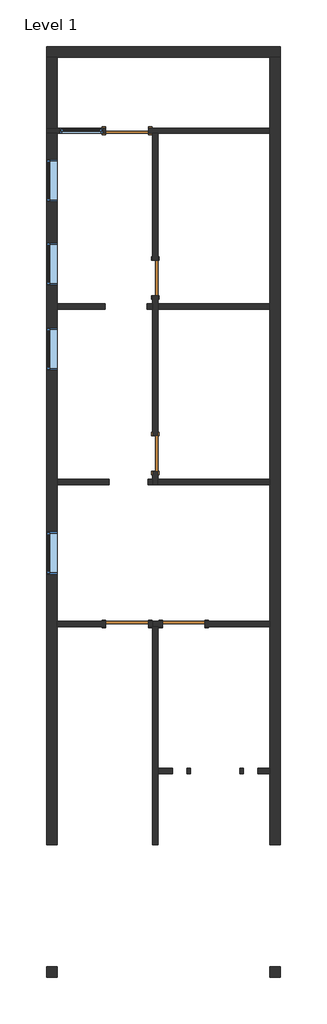
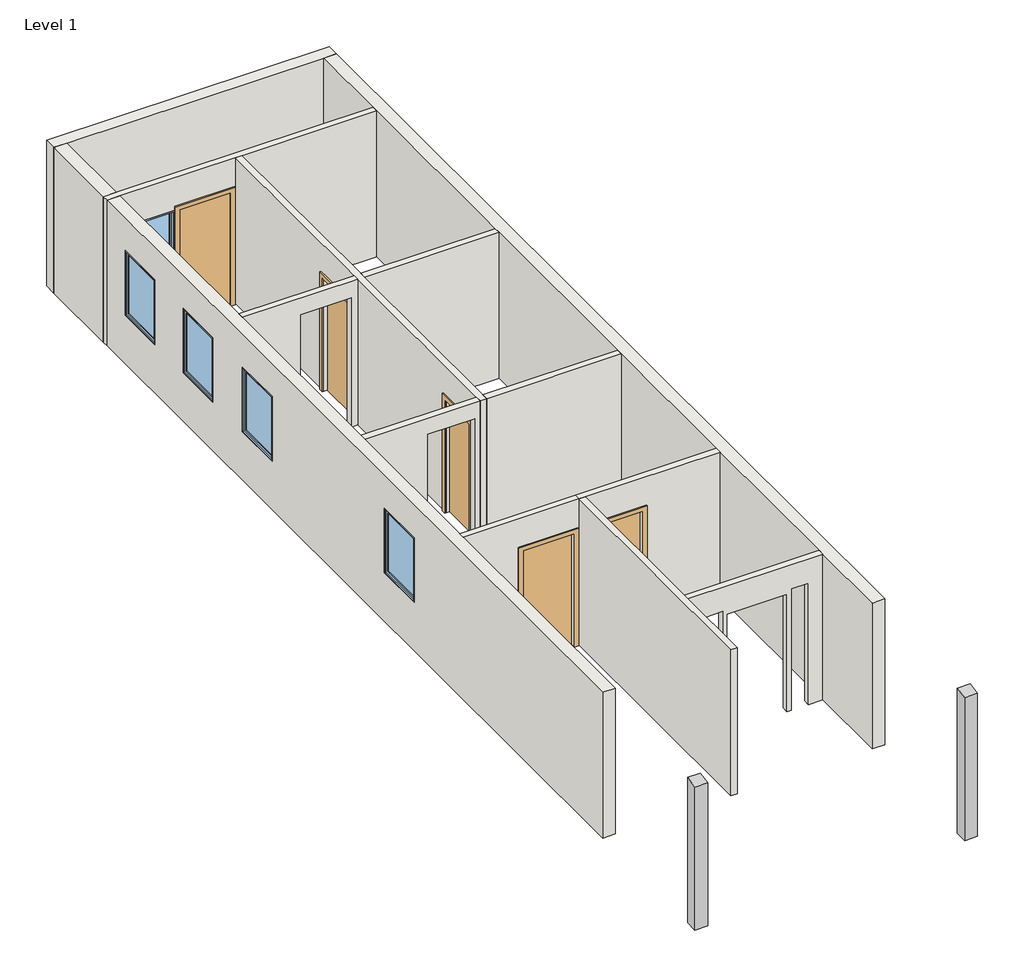
# One storey, incomplete: 14 walls, 5 doors, 5 windows, 2 columns.
"""IFC4 building model written with IfcOpenShell, lengths in millimetres."""

from ifc_helpers import new_model, si_unit, point, frame, frame_2d, origin, origin_with_axes, place, context, project, spatial, polyline, circle_curve, trimmed, segment, composite_curve, outline, extrude, faceted_brep, transform, mapped, element, save
from components import door_214872d5, door_305aa2a5, window_c1f32544, window_41a96561

model = new_model("IFC4")

# Units and contexts
model_context = context("Model", 3, world=origin())
ifc_project = project(units=[si_unit("LENGTHUNIT", "METRE", prefix="MILLI")], contexts=[model_context])

# Site, building, storey
site = spatial("IfcSite", under=ifc_project)
building = spatial("IfcBuilding", under=site)
storey = spatial("IfcBuildingStorey", under=building, Name="Level 1", Elevation=0.0)

# Columns
placement = place(None, origin())
element("IfcColumn", 1, ObjectType="Rectangular Column : 9\"X9\"", at=placement, inside=storey, context=model_context, shape_type="SweptSolid", body=[
    extrude(outline(composite_curve([segment(polyline([(-16023.0597562, 0.0), (-16251.6597562, 0.0), (-16251.6597562, 2691.3651661)]), True, "CONTINUOUS"), segment(trimmed(circle_curve(frame_2d((-13694.3342361, -9875.5261928)), 12824.4560213), [point((-16251.6597562, 2691.3651661))], [point((-16023.0597562, 2735.7271031))], False, "CARTESIAN"), True, "CONTINUOUS"), segment(polyline([(-16023.0597562, 2735.7271031), (-16023.0597562, 0.0)]), True, "CONTINUOUS")], self_intersect=False)), frame((-5651.4766939, 0.0, 0.0), z_axis=(1.0, 0.0, 0.0), x_axis=(0.0, 1.0, 0.0)), (0.0, 0.0, 1.0), 228.6),
])
element("IfcColumn", 2, ObjectType="Rectangular Column : 9\"X9\"", at=placement, inside=storey, context=model_context, shape_type="SweptSolid", body=[
    extrude(outline(composite_curve([segment(polyline([(-16023.0597562, 0.0), (-16251.6597562, 0.0), (-16251.6597562, 2691.3651661)]), True, "CONTINUOUS"), segment(trimmed(circle_curve(frame_2d((-13694.3342361, -9875.5261928)), 12824.4560213), [point((-16251.6597562, 2691.3651661))], [point((-16023.0597562, 2735.7271031))], False, "CARTESIAN"), True, "CONTINUOUS"), segment(polyline([(-16023.0597562, 2735.7271031), (-16023.0597562, 0.0)]), True, "CONTINUOUS")], self_intersect=False)), frame((-850.8766939, 0.0, 0.0), z_axis=(1.0, 0.0, 0.0), x_axis=(0.0, 1.0, 0.0)), (0.0, 0.0, 1.0), 228.6),
])

# Doors
door_shape = door_214872d5(model_context)
element("IfcDoor", 3, ObjectType="Single-Flush : 30\" x 84\"", at=placement, inside=storey, context=model_context, shape_type="MappedRepresentation", body=[
    mapped(door_shape, transform((-3308.3266939, -4999.4597562, 0.0), x_axis=(0.0, -1.0, 0.0), y_axis=(1.0, 0.0, 0.0), z_axis=(0.0, 0.0, 1.0))),
])
element("IfcDoor", 4, ObjectType="Single-Flush : 30\" x 84\"", at=placement, inside=storey, context=model_context, shape_type="MappedRepresentation", body=[
    mapped(door_shape, transform((-3308.3266939, -1227.5597562, 0.0), x_axis=(0.0, -1.0, 0.0), y_axis=(1.0, 0.0, 0.0), z_axis=(0.0, 0.0, 1.0))),
])
door_2_shape = door_305aa2a5(model_context)
element("IfcDoor", 5, ObjectType="Single-Flush : 36\" x 84\"", at=placement, inside=storey, context=model_context, shape_type="MappedRepresentation", body=[
    mapped(door_2_shape, transform((-3917.9266939, -8657.0597562, 0.0), x_axis=(-1.0, 0.0, 0.0), y_axis=(0.0, -1.0, 0.0), z_axis=(0.0, 0.0, 1.0))),
])
element("IfcDoor", 6, ObjectType="Single-Flush : 36\" x 84\"", at=placement, inside=storey, context=model_context, shape_type="MappedRepresentation", body=[
    mapped(door_2_shape, transform((-2698.7266939, -8657.0597562, 0.0), x_axis=(-1.0, 0.0, 0.0), y_axis=(0.0, -1.0, 0.0), z_axis=(0.0, 0.0, 1.0))),
])
element("IfcDoor", 7, ObjectType="Single-Flush : 36\" x 84\"", at=placement, inside=storey, context=model_context, shape_type="MappedRepresentation", body=[
    mapped(door_2_shape, transform((-3917.9266939, 1934.7402438, 0.0), x_axis=(1.0, 0.0, 0.0), y_axis=(0.0, 1.0, 0.0), z_axis=(0.0, 0.0, 1.0))),
])

# Walls
element("IfcWall", 8, ObjectType="wall 4.5\"", at=placement, inside=storey, context=model_context, shape_type="Brep", body=[
    faceted_brep([(-850.8766939, 1991.8902438, 0.0), (-3460.7266939, 1991.8902438, 0.0), (-3460.7266939, 1991.8902438, 2133.6), (-4375.1266939, 1991.8902438, 2133.6), (-4375.1266939, 1991.8902438, 0.0), (-5422.8766939, 1991.8902438, 0.0), (-5651.4766939, 1991.8902438, 0.0), (-5651.4766939, 1991.8902438, 2743.2), (-5422.8766939, 1991.8902438, 2743.2), (-850.8766939, 1991.8902438, 2743.2), (-4444.9766939, 1991.8902438, 2133.6), (-5359.3766939, 1991.8902438, 2133.6), (-5359.3766939, 1991.8902438, 914.4), (-4444.9766939, 1991.8902438, 914.4), (-3460.7266939, 1877.5902438, 2133.6), (-3460.7266939, 1877.5902438, 0.0), (-3365.4766939, 1877.5902438, 0.0), (-3251.1766939, 1877.5902438, 0.0), (-850.8766939, 1877.5902438, 0.0), (-850.8766939, 1877.5902438, 2743.2), (-3251.1766939, 1877.5902438, 2743.2), (-3365.4766939, 1877.5902438, 2743.2), (-5422.8766939, 1877.5902438, 2743.2), (-5651.4766939, 1877.5902438, 2743.2), (-5651.4766939, 1877.5902438, 0.0), (-5422.8766939, 1877.5902438, 0.0), (-4375.1266939, 1877.5902438, 0.0), (-4375.1266939, 1877.5902438, 2133.6), (-4444.9766939, 1877.5902438, 2133.6), (-4444.9766939, 1877.5902438, 914.4), (-5359.3766939, 1877.5902438, 914.4), (-5359.3766939, 1877.5902438, 2133.6)], [[[0, 1, 2, 3, 4, 5, 6, 7, 8, 9], [10, 11, 12, 13]], [[14, 15, 16, 17, 18, 19, 20, 21, 22, 23, 24, 25, 26, 27], [28, 29, 30, 31]], [[26, 25, 24, 6, 5, 4]], [[18, 17, 16, 15, 1, 0]], [[0, 9, 19, 18]], [[7, 6, 24, 23]], [[2, 1, 15, 14]], [[3, 2, 14, 27]], [[4, 3, 27, 26]], [[29, 28, 10, 13]], [[30, 29, 13, 12]], [[31, 30, 12, 11]], [[28, 31, 11, 10]], [[9, 8, 7, 23, 22, 21, 20, 19]]]),
])
element("IfcWall", 9, ObjectType="wall 4.5\"", at=placement, inside=storey, context=model_context, shape_type="Brep", body=[
    faceted_brep([(-3365.4766939, -1608.5597562, 2133.6), (-3365.4766939, -1608.5597562, 0.0), (-3365.4766939, -1780.0097562, 0.0), (-3365.4766939, -1894.3097562, 0.0), (-3365.4766939, -4618.4597562, 0.0), (-3365.4766939, -4618.4597562, 2133.6), (-3365.4766939, -5380.4597562, 2133.6), (-3365.4766939, -5380.4597562, 0.0), (-3365.4766939, -5551.9097562, 0.0), (-3365.4766939, -5666.2097562, 0.0), (-3365.4766939, -5666.2097562, 2743.2), (-3365.4766939, -5551.9097562, 2743.2), (-3365.4766939, -1894.3097562, 2743.2), (-3365.4766939, -1780.0097562, 2743.2), (-3365.4766939, 1877.5902438, 2743.2), (-3365.4766939, 1877.5902438, 0.0), (-3365.4766939, -846.5597562, 0.0), (-3365.4766939, -846.5597562, 2133.6), (-3251.1766939, -4618.4597562, 0.0), (-3251.1766939, -1894.3097562, 0.0), (-3251.1766939, -1780.0097562, 0.0), (-3251.1766939, -1608.5597562, 0.0), (-3251.1766939, -1608.5597562, 2133.6), (-3251.1766939, -846.5597562, 2133.6), (-3251.1766939, -846.5597562, 0.0), (-3251.1766939, 1877.5902438, 0.0), (-3251.1766939, 1877.5902438, 2743.2), (-3251.1766939, -1780.0097562, 2743.2), (-3251.1766939, -1894.3097562, 2743.2), (-3251.1766939, -5551.9097562, 2743.2), (-3251.1766939, -5666.2097562, 2743.2), (-3251.1766939, -5666.2097562, 0.0), (-3251.1766939, -5551.9097562, 0.0), (-3251.1766939, -5380.4597562, 0.0), (-3251.1766939, -5380.4597562, 2133.6), (-3251.1766939, -4618.4597562, 2133.6)], [[[0, 1, 2, 3, 4, 5, 6, 7, 8, 9, 10, 11, 12, 13, 14, 15, 16, 17]], [[18, 19, 20, 21, 22, 23, 24, 25, 26, 27, 28, 29, 30, 31, 32, 33, 34, 35]], [[9, 8, 7, 33, 32, 31]], [[16, 15, 25, 24]], [[4, 3, 2, 1, 21, 20, 19, 18]], [[15, 14, 26, 25]], [[10, 9, 31, 30]], [[34, 33, 7, 6]], [[35, 34, 6, 5]], [[18, 35, 5, 4]], [[22, 21, 1, 0]], [[23, 22, 0, 17]], [[24, 23, 17, 16]], [[14, 13, 12, 11, 10, 30, 29, 28, 27, 26]]]),
])
element("IfcWall", 10, ObjectType="wall 4.5\"", at=placement, inside=storey, context=model_context, shape_type="SweptSolid", body=[
    extrude(outline(polyline([(-850.8766939, -1894.3097562), (-3251.1766939, -1894.3097562), (-3251.1766939, -1780.0097562), (-850.8766939, -1780.0097562), (-850.8766939, -1894.3097562)])), origin_with_axes(), (0.0, 0.0, 1.0), 2743.2),
])
element("IfcWall", 11, ObjectType="wall 4.5\"", at=placement, inside=storey, context=model_context, shape_type="SweptSolid", body=[
    extrude(outline(polyline([(-850.8766939, -5666.2097562), (-3251.1766939, -5666.2097562), (-3251.1766939, -5551.9097562), (-850.8766939, -5551.9097562), (-850.8766939, -5666.2097562)])), origin_with_axes(), (0.0, 0.0, 1.0), 2743.2),
])
element("IfcWall", 12, ObjectType="wall 4.5\"", at=placement, inside=storey, context=model_context, shape_type="Brep", body=[
    faceted_brep([(-3365.4766939, -8714.2097562, 0.0), (-3251.1766939, -8714.2097562, 0.0), (-3155.9266939, -8714.2097562, 0.0), (-3155.9266939, -8714.2097562, 2133.6), (-2241.5266939, -8714.2097562, 2133.6), (-2241.5266939, -8714.2097562, 0.0), (-850.8766939, -8714.2097562, 0.0), (-850.8766939, -8714.2097562, 2743.2), (-3251.1766939, -8714.2097562, 2743.2), (-3365.4766939, -8714.2097562, 2743.2), (-3155.9266939, -8599.9097562, 2133.6), (-3155.9266939, -8599.9097562, 0.0), (-3365.4766939, -8599.9097562, 0.0), (-3365.4766939, -8599.9097562, 2743.2), (-850.8766939, -8599.9097562, 2743.2), (-850.8766939, -8599.9097562, 0.0), (-2241.5266939, -8599.9097562, 0.0), (-2241.5266939, -8599.9097562, 2133.6)], [[[0, 1, 2, 3, 4, 5, 6, 7, 8, 9]], [[10, 11, 12, 13, 14, 15, 16, 17]], [[16, 15, 6, 5]], [[12, 11, 2, 1, 0]], [[7, 6, 15, 14]], [[3, 2, 11, 10]], [[4, 3, 10, 17]], [[5, 4, 17, 16]], [[0, 9, 13, 12]], [[9, 8, 7, 14, 13]]]),
])
element("IfcWall", 13, ObjectType="wall 4.5\"", at=placement, inside=storey, context=model_context, shape_type="SweptSolid", body=[
    extrude(outline(polyline([(0.0, -1489.0516939), (0.0, -1412.8516939), (2286.0, -1412.8516939), (2286.0, -1108.0516939), (0.0, -1108.0516939), (0.0, -850.8766939), (2743.2, -850.8766939), (2743.2, -3251.1766939), (0.0, -3251.1766939), (0.0, -2936.8516939), (2286.0, -2936.8516939), (2286.0, -2632.0516939), (0.0, -2632.0516939), (0.0, -2555.8516939), (2209.8, -2555.8516939), (2209.8, -1489.0516939), (0.0, -1489.0516939)])), frame((0.0, -11876.5097562, 0.0), z_axis=(0.0, 1.0, 0.0), x_axis=(0.0, 0.0, 1.0)), (0.0, 0.0, 1.0), 114.3),
])
element("IfcWall", 14, ObjectType="wall 4.5\"", at=placement, inside=storey, context=model_context, shape_type="SweptSolid", body=[
    extrude(outline(polyline([(2743.2, -5422.8766939), (0.0, -5422.8766939), (0.0, -4391.959165), (2438.4, -4391.959165), (2438.4, -3483.8028016), (0.0, -3483.8028016), (0.0, -3365.4766939), (2743.2, -3365.4766939), (2743.2, -5422.8766939)])), frame((0.0, -1894.3097562, 0.0), z_axis=(0.0, 1.0, 0.0), x_axis=(0.0, 0.0, 1.0)), (0.0, 0.0, 1.0), 114.3),
])
element("IfcWall", 15, ObjectType="wall 4.5\"", at=placement, inside=storey, context=model_context, shape_type="SweptSolid", body=[
    extrude(outline(polyline([(2743.2, -5422.8766939), (0.0, -5422.8766939), (0.0, -4303.9674393), (2438.4, -4303.9674393), (2438.4, -3463.2909707), (0.0, -3463.2909707), (0.0, -3365.4766939), (2743.2, -3365.4766939), (2743.2, -5422.8766939)])), frame((0.0, -5666.2097562, 0.0), z_axis=(0.0, 1.0, 0.0), x_axis=(0.0, 0.0, 1.0)), (0.0, 0.0, 1.0), 114.3),
])
element("IfcWall", 16, ObjectType="wall 4.5\"", at=placement, inside=storey, context=model_context, shape_type="SweptSolid", body=[
    extrude(outline(polyline([(0.0, -5422.8766939), (0.0, -4375.1266939), (2133.6, -4375.1266939), (2133.6, -3460.7266939), (0.0, -3460.7266939), (0.0, -3365.4766939), (2743.2, -3365.4766939), (2743.2, -5422.8766939), (0.0, -5422.8766939)])), frame((0.0, -8714.2097562, 0.0), z_axis=(0.0, 1.0, 0.0), x_axis=(0.0, 0.0, 1.0)), (0.0, 0.0, 1.0), 114.3),
])
element("IfcWall", 17, ObjectType="wall 4.5\"", at=placement, inside=storey, context=model_context, shape_type="Brep", body=[
    faceted_brep([(-3365.4766939, -8714.2097562, 0.0), (-3365.4766939, -13400.5097562, 0.0), (-3365.4766939, -13400.5097562, 2743.2), (-3365.4766939, -8714.2097562, 2743.2), (-3251.1766939, -8714.2097562, 0.0), (-3251.1766939, -8714.2097562, 2743.2), (-3251.1766939, -11762.2097562, 2743.2), (-3251.1766939, -11876.5097562, 2743.2), (-3251.1766939, -13400.5097562, 2743.2), (-3251.1766939, -13400.5097562, 0.0), (-3251.1766939, -11876.5097562, 0.0), (-3251.1766939, -11762.2097562, 0.0)], [[[0, 1, 2, 3]], [[4, 5, 6, 7, 8, 9, 10, 11]], [[1, 0, 4, 11, 10, 9]], [[2, 1, 9, 8]], [[0, 3, 5, 4]], [[3, 2, 8, 7, 6, 5]]]),
])
element("IfcWall", 18, ObjectType="wall 9\"", at=placement, inside=storey, context=model_context, shape_type="Brep", body=[
    faceted_brep([(-5651.4766939, 3515.8902438, 0.0), (-5422.8766939, 3515.8902438, 0.0), (-850.8766939, 3515.8902438, 0.0), (-622.2766939, 3515.8902438, 0.0), (-622.2766939, 3515.8902438, 2743.2), (-850.8766939, 3515.8902438, 2743.2), (-5422.8766939, 3515.8902438, 2743.2), (-5651.4766939, 3515.8902438, 2743.2), (-5651.4766939, 3744.4902438, 0.0), (-5651.4766939, 3744.4902438, 2743.2), (-622.2766939, 3744.4902438, 2743.2), (-622.2766939, 3744.4902438, 0.0)], [[[0, 1, 2, 3, 4, 5, 6, 7]], [[8, 9, 10, 11]], [[3, 2, 1, 0, 8, 11]], [[4, 3, 11, 10]], [[0, 7, 9, 8]], [[7, 6, 5, 4, 10, 9]]]),
])
element("IfcWall", 19, ObjectType="wall 9\"", at=placement, inside=storey, context=model_context, shape_type="Brep", body=[
    faceted_brep([(-850.8766939, 3515.8902438, 0.0), (-850.8766939, 1991.8902438, 0.0), (-850.8766939, 1877.5902438, 0.0), (-850.8766939, -1780.0097562, 0.0), (-850.8766939, -1894.3097562, 0.0), (-850.8766939, -5551.9097562, 0.0), (-850.8766939, -5666.2097562, 0.0), (-850.8766939, -8599.9097562, 0.0), (-850.8766939, -8714.2097562, 0.0), (-850.8766939, -11762.2097562, 0.0), (-850.8766939, -11876.5097562, 0.0), (-850.8766939, -13400.5097562, 0.0), (-850.8766939, -13400.5097562, 2743.2), (-850.8766939, -11876.5097562, 2743.2), (-850.8766939, -11762.2097562, 2743.2), (-850.8766939, -8714.2097562, 2743.2), (-850.8766939, -8599.9097562, 2743.2), (-850.8766939, -5666.2097562, 2743.2), (-850.8766939, -5551.9097562, 2743.2), (-850.8766939, -1894.3097562, 2743.2), (-850.8766939, -1780.0097562, 2743.2), (-850.8766939, 1877.5902438, 2743.2), (-850.8766939, 1991.8902438, 2743.2), (-850.8766939, 3515.8902438, 2743.2), (-622.2766939, 3515.8902438, 0.0), (-622.2766939, 3515.8902438, 2743.2), (-622.2766939, -13400.5097562, 2743.2), (-622.2766939, -13400.5097562, 0.0)], [[[0, 1, 2, 3, 4, 5, 6, 7, 8, 9, 10, 11, 12, 13, 14, 15, 16, 17, 18, 19, 20, 21, 22, 23]], [[24, 25, 26, 27]], [[11, 10, 9, 8, 7, 6, 5, 4, 3, 2, 1, 0, 24, 27]], [[12, 11, 27, 26]], [[0, 23, 25, 24]], [[23, 22, 21, 20, 19, 18, 17, 16, 15, 14, 13, 12, 26, 25]]]),
])
element("IfcWall", 20, ObjectType="wall 9\"", at=placement, inside=storey, context=model_context, shape_type="SweptSolid", body=[
    extrude(outline(polyline([(-5651.4766939, 1991.8902438), (-5651.4766939, 3515.8902438), (-5422.8766939, 3515.8902438), (-5422.8766939, 1991.8902438), (-5651.4766939, 1991.8902438)])), origin_with_axes(), (0.0, 0.0, 1.0), 2743.2),
])
element("IfcWall", 21, ObjectType="wall 9\"", at=placement, inside=storey, context=model_context, shape_type="Brep", body=[
    faceted_brep([(-5422.8766939, -13400.5097562, 0.0), (-5422.8766939, -8714.2097562, 0.0), (-5422.8766939, -8599.9097562, 0.0), (-5422.8766939, -5666.2097562, 0.0), (-5422.8766939, -5551.9097562, 0.0), (-5422.8766939, -1894.3097562, 0.0), (-5422.8766939, -1780.0097562, 0.0), (-5422.8766939, 1877.5902438, 0.0), (-5422.8766939, 1877.5902438, 2743.2), (-5422.8766939, -1780.0097562, 2743.2), (-5422.8766939, -1894.3097562, 2743.2), (-5422.8766939, -5551.9097562, 2743.2), (-5422.8766939, -5666.2097562, 2743.2), (-5422.8766939, -8599.9097562, 2743.2), (-5422.8766939, -8714.2097562, 2743.2), (-5422.8766939, -13400.5097562, 2743.2), (-5422.8766939, -6675.8597562, 2133.6), (-5422.8766939, -6675.8597562, 914.4), (-5422.8766939, -7590.2597562, 914.4), (-5422.8766939, -7590.2597562, 2133.6), (-5422.8766939, -2294.3597562, 2133.6), (-5422.8766939, -2294.3597562, 914.4), (-5422.8766939, -3208.7597562, 914.4), (-5422.8766939, -3208.7597562, 2133.6), (-5422.8766939, 1325.1402438, 2133.6), (-5422.8766939, 1325.1402438, 914.4), (-5422.8766939, 410.7402438, 914.4), (-5422.8766939, 410.7402438, 2133.6), (-5422.8766939, -465.5597562, 2133.6), (-5422.8766939, -465.5597562, 914.4), (-5422.8766939, -1379.9597562, 914.4), (-5422.8766939, -1379.9597562, 2133.6), (-5651.4766939, -13400.5097562, 0.0), (-5651.4766939, -13400.5097562, 2743.2), (-5651.4766939, 1877.5902438, 2743.2), (-5651.4766939, 1877.5902438, 0.0), (-5651.4766939, -6675.8597562, 2133.6), (-5651.4766939, -7590.2597562, 2133.6), (-5651.4766939, -7590.2597562, 914.4), (-5651.4766939, -6675.8597562, 914.4), (-5651.4766939, -2294.3597562, 2133.6), (-5651.4766939, -3208.7597562, 2133.6), (-5651.4766939, -3208.7597562, 914.4), (-5651.4766939, -2294.3597562, 914.4), (-5651.4766939, 1325.1402438, 2133.6), (-5651.4766939, 410.7402438, 2133.6), (-5651.4766939, 410.7402438, 914.4), (-5651.4766939, 1325.1402438, 914.4), (-5651.4766939, -465.5597562, 2133.6), (-5651.4766939, -1379.9597562, 2133.6), (-5651.4766939, -1379.9597562, 914.4), (-5651.4766939, -465.5597562, 914.4)], [[[0, 1, 2, 3, 4, 5, 6, 7, 8, 9, 10, 11, 12, 13, 14, 15], [16, 17, 18, 19], [20, 21, 22, 23], [24, 25, 26, 27], [28, 29, 30, 31]], [[32, 33, 34, 35], [36, 37, 38, 39], [40, 41, 42, 43], [44, 45, 46, 47], [48, 49, 50, 51]], [[7, 6, 5, 4, 3, 2, 1, 0, 32, 35]], [[0, 15, 33, 32]], [[8, 7, 35, 34]], [[17, 16, 36, 39]], [[18, 17, 39, 38]], [[19, 18, 38, 37]], [[16, 19, 37, 36]], [[21, 20, 40, 43]], [[22, 21, 43, 42]], [[23, 22, 42, 41]], [[20, 23, 41, 40]], [[25, 24, 44, 47]], [[26, 25, 47, 46]], [[27, 26, 46, 45]], [[24, 27, 45, 44]], [[29, 28, 48, 51]], [[30, 29, 51, 50]], [[31, 30, 50, 49]], [[28, 31, 49, 48]], [[15, 14, 13, 12, 11, 10, 9, 8, 34, 33]]]),
])

# Windows
window_shape = window_c1f32544(model_context)
element("IfcWindow", 22, ObjectType="Fixed : 36\" x 48\"", at=placement, inside=storey, context=model_context, shape_type="MappedRepresentation", body=[
    mapped(window_shape, transform((-5537.1766939, -7094.9597562, 0.0), x_axis=(0.0, 1.0, 0.0), y_axis=(-1.0, 0.0, 0.0), z_axis=(0.0, 0.0, 1.0))),
])
element("IfcWindow", 23, ObjectType="Fixed : 36\" x 48\"", at=placement, inside=storey, context=model_context, shape_type="MappedRepresentation", body=[
    mapped(window_shape, transform((-5537.1766939, -2713.4597562, 0.0), x_axis=(0.0, 1.0, 0.0), y_axis=(-1.0, 0.0, 0.0), z_axis=(0.0, 0.0, 1.0))),
])
element("IfcWindow", 24, ObjectType="Fixed : 36\" x 48\"", at=placement, inside=storey, context=model_context, shape_type="MappedRepresentation", body=[
    mapped(window_shape, transform((-5537.1766939, 906.0402438, 0.0), x_axis=(0.0, 1.0, 0.0), y_axis=(-1.0, 0.0, 0.0), z_axis=(0.0, 0.0, 1.0))),
])
element("IfcWindow", 25, ObjectType="Fixed : 36\" x 48\"", at=placement, inside=storey, context=model_context, shape_type="MappedRepresentation", body=[
    mapped(window_shape, transform((-5537.1766939, -884.6597562, 0.0), x_axis=(0.0, 1.0, 0.0), y_axis=(-1.0, 0.0, 0.0), z_axis=(0.0, 0.0, 1.0))),
])
window_2_shape = window_41a96561(model_context)
element("IfcWindow", 26, ObjectType="Fixed : 36\" x 48\"", at=placement, inside=storey, context=model_context, shape_type="MappedRepresentation", body=[
    mapped(window_2_shape, transform((-4864.0766939, 1934.7402438, 0.0), x_axis=(1.0, 0.0, 0.0), y_axis=(0.0, 1.0, 0.0), z_axis=(0.0, 0.0, 1.0))),
])

save(model, "model.ifc")

# Revit data of these elements
# Type "Rectangular Column : 9\"X9\""
#   Assembly Code = "B1010200"
#   Depth = 0' - 9"
#   Offset Base = 0' - 0"
#   Offset Top = 0' - 0"
#   Width = 0' - 9"
#   Material = none
# Type "Single-Flush : 30\" x 84\""
#   Type Mark = "4"
#   Construction Type Id = "MDOOR"
#   Assembly Code = "C1020"
#   Analytic Construction = "Metal"
#   Thickness = 0' - 2"
#   Heat Transfer Coefficient (U) = 0.651978 BTU/(h·ft²·°F)
#   Height = 7' - 0"
#   Trim Projection Ext = 0' - 1"
#   Trim Projection Int = 0' - 1"
#   Trim Width = 0' - 3"
#   Width = 2' - 6"
#   Define Thermal Properties by = 1
#   Define Thermal Properties by = 1
#   Door Material = Door - Panel
#   Frame Material = Door - Frame
#   Visual Light Transmittance = 0
#   Solar Heat Gain Coefficient = 0
#   Function = (empty or 0)
#   Wall Closure = (empty or 0)
# Type "Single-Flush : 36\" x 84\""
#   Type Mark = "1"
#   Construction Type Id = "MDOOR"
#   Assembly Code = "C1020"
#   Analytic Construction = "Metal"
#   Thickness = 0' - 2"
#   Heat Transfer Coefficient (U) = 0.651978 BTU/(h·ft²·°F)
#   Height = 7' - 0"
#   Trim Projection Ext = 0' - 1"
#   Trim Projection Int = 0' - 1"
#   Trim Width = 0' - 3"
#   Width = 3' - 0"
#   Define Thermal Properties by = 1
#   Define Thermal Properties by = 1
#   Door Material = Door - Panel
#   Frame Material = Door - Frame
#   Visual Light Transmittance = 0
#   Solar Heat Gain Coefficient = 0
#   Function = (empty or 0)
#   Wall Closure = (empty or 0)
# Type "wall 4.5\""
#   Assembly Code = "B2010"
#   Layers, outside or top first: 0' - 4 1/2" no material (function 1)
# Type "wall 9\""
#   Assembly Code = "B2010"
#   Layers, outside or top first: 0' - 9" no material (function 1)
# Type "Fixed : 36\" x 48\""
#   Type Mark = "1"
#   Construction Type Id = "GSP4R"
#   Assembly Code = "B2020100"
#   Analytic Construction = "1/8 in Pilkington single glazing"
#   Visual Light Transmittance = 0.9
#   Solar Heat Gain Coefficient = 0.78
#   Heat Transfer Coefficient (U) = 0.6496 BTU/(h·ft²·°F)
#   Height = 4' - 0"
#   Default Sill Height = 3' - 0"
#   Width = 3' - 0"
#   Window Inset = 0' - 0 3/4"
#   Define Thermal Properties by = 1
#   Define Thermal Properties by = 1
#   Glass Pane Material = Glass
#   Sash Material = Sash
#   Wall Closure = (empty or 0)
# Elements 1, 2 (IfcColumn, "Rectangular Column : 9\"X9\"")
#   Phase Created = New Construction
# Elements 3, 4 (IfcDoor, "Single-Flush : 30\" x 84\"")
#   Phase Created = New Construction
#   Materials on its faces: "Door - Frame", "Door - Panel"
# Elements 5, 6, 7 (IfcDoor, "Single-Flush : 36\" x 84\"")
#   Phase Created = New Construction
#   Materials on its faces: "Door - Frame", "Door - Panel"
# Elements 8, 9, 10, 11, 12, 13, 14, 15, 16, 17 (IfcWall, "wall 4.5\"")
#   Top Offset = 0' - 0"
#   Base Offset = 0' - 0"
#   wall height = 9' - 0"
#   Phase Created = New Construction
#   Base Constraint = Level 1
#   Top Constraint = Level 2
#   Materials on its faces: "Default Wall"
# Elements 18, 19, 20, 21 (IfcWall, "wall 9\"")
#   Top Offset = 0' - 0"
#   Base Offset = 0' - 0"
#   wall height = 9' - 0"
#   Phase Created = New Construction
#   Base Constraint = Level 1
#   Top Constraint = Level 2
#   Materials on its faces: "Default Wall"
# Element 22 (IfcWindow, "Fixed : 36\" x 48\"")
#   Mark = "1"
#   Phase Created = New Construction
#   Materials on its faces: "Sash", "Glass"
# Element 23 (IfcWindow, "Fixed : 36\" x 48\"")
#   Mark = "2"
#   Phase Created = New Construction
#   Materials on its faces: "Sash", "Glass"
# Element 24 (IfcWindow, "Fixed : 36\" x 48\"")
#   Mark = "3"
#   Phase Created = New Construction
#   Materials on its faces: "Sash", "Glass"
# Element 25 (IfcWindow, "Fixed : 36\" x 48\"")
#   Mark = "4"
#   Phase Created = New Construction
#   Materials on its faces: "Sash", "Glass"
# Element 26 (IfcWindow, "Fixed : 36\" x 48\"")
#   Mark = "5"
#   Phase Created = New Construction
#   Materials on its faces: "Sash", "Glass"
# Materials
#   "Door - Panel": class "Wood", colour RGB 210 159 95, transparency 0, Cost = 0
#   "Door - Frame": colour RGB 118 70 51, transparency 0, Cost = 0
#   "Glass": class "Glass", colour RGB 0 128 192, transparency 0.75, Description = "Soda Lime Glass", Cost = 0
#   "Sash": class "Wood", colour RGB 224 178 126, transparency 0, Cost = 0
#   "Default Wall": colour RGB 128 128 128, transparency 0, Cost = 0
